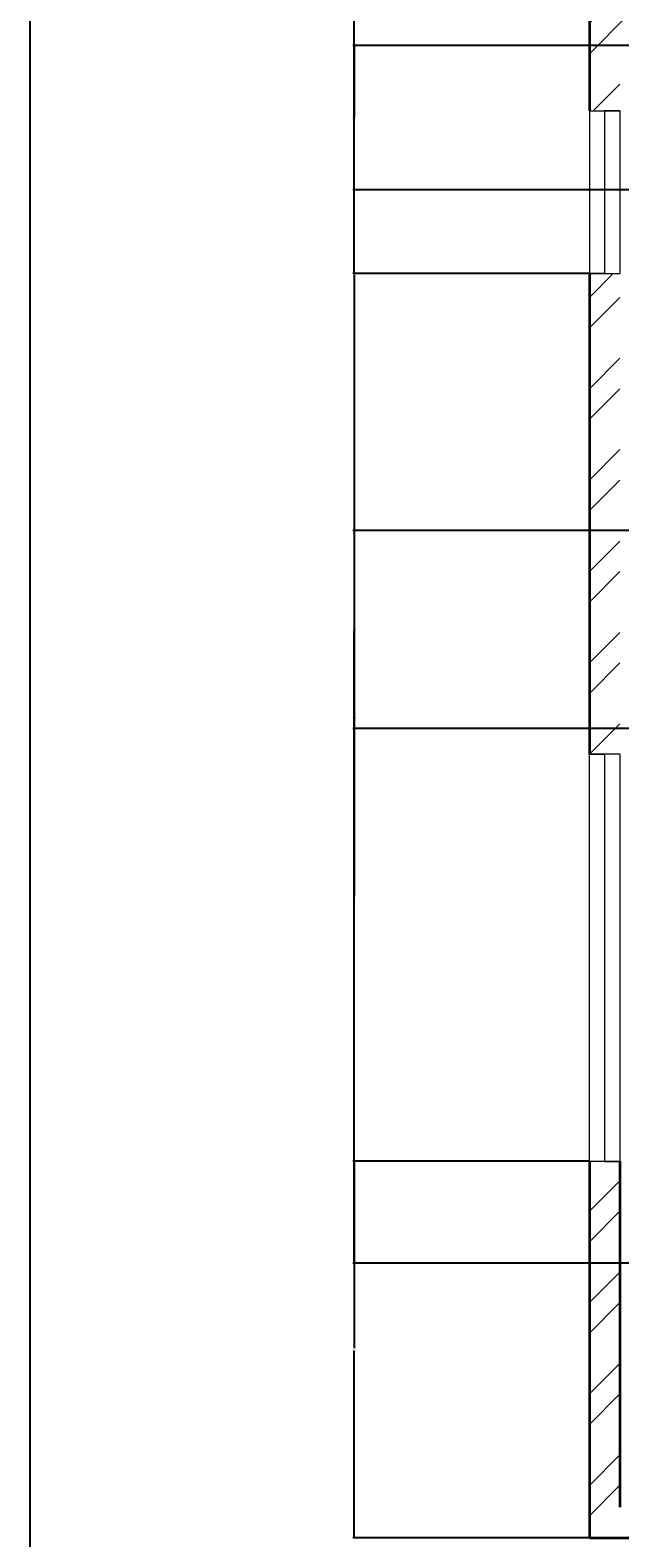
# Model space of a CAD drawing. Units: inches. Extents: x 1965 to 2673, y 1802 to 2669.
# Tile 2 of 16: x 1965 to 2052, y 1932 to 2154. Entities that reach past the tile are written whole.
import ezdxf

# ---------------------------------------------------------------- set-up
doc = ezdxf.new("R2010")
doc.units = ezdxf.units.IN
for name, color, linetype, lineweight in [('A-ANNO-DIMS', 2, 'Continuous', 18), ('A-ANNO-TTLB', 7, 'Continuous', 25), ('A-GLAZ', 181, 'Continuous', 18), ('A-WALL', 7, 'Continuous', 35), ('A-WALL-PATT', 252, 'Continuous', 13)]:
    doc.layers.add(name, color=color, linetype=linetype, lineweight=lineweight)
doc.styles.get("Standard").update_dxf_attribs({"font": 'arial.ttf'})
doc.dimstyles.get("Standard").update_dxf_attribs({"dimtxt": 0.18, "dimasz": 0.18, "dimexe": 0.18, "dimexo": 0.0625, "dimgap": 0.09, "dimtad": 0, "dimtih": 1, "dimtoh": 1, "dimdec": 4, "dimzin": 0, "dimdsep": 46, "dimtxsty": 'Standard', "dimcen": 0.09, "dimadec": 0, "dimazin": 0, "dimtfac": 1, "dimtdec": 4, "dimtofl": 0, "dimtmove": 0, "dimatfit": 3, "dimfxl": 1, "dimtolj": 1, "dimtzin": 0, "dimarcsym": 0})

# ---------------------------------------------------------------- blocks, each defined once
blk = doc.blocks.new('WIN-60IN')
for p, q in [((0, 4.5), (0, 0)), ((0, 4.5), (60, 4.5)), ((60, 2.25), (60, 4.5)), ((60, 4.5), (60, 0)), ((0, 0), (0, 2.25)), ((0, 2.25), (60, 2.25)), ((60, 0), (0, 0))]:
    blk.add_line(p, q)
blk = doc.blocks.new('WIN-24IN')
for p, q in [((0, 24), (4.5, 24)), ((0, 24), (0, 0)), ((4.5, 24), (2.25, 24)), ((2.25, 24), (2.25, 0)), ((4.5, 24), (4.5, 0)), ((2.25, 0), (0, 0)), ((0, 0), (4.5, 0))]:
    blk.add_line(p, q)
blk = doc.blocks.new('*D33')
at = {"layer": 'A-ANNO-DIMS', "color": 0, "lineweight": -2, "transparency": 16777216}
for p, q in [((2047.03, 1987.1), (2012.19, 1987.1)), ((2012.37, 1986.92), (2012.37, 1959.53)), ((2012.37, 1931.77), (2012.37, 1959.16)), ((2047.03, 1931.59), (2012.19, 1931.59))]:
    blk.add_line(p, q, dxfattribs=at)
at = {"layer": 'A-ANNO-DIMS', "color": 0, "transparency": 16777216}
for points in [[(2012.34, 1986.92), (2012.4, 1986.92), (2012.37, 1987.1)], [(2012.34, 1931.77), (2012.4, 1931.77), (2012.37, 1931.59)]]:
    blk.add_solid(points, dxfattribs=at)
at = {"layer": 'Defpoints', "color": 0, "transparency": 16777216}
for p in [(2012.37, 1987.1), (2047.09, 1987.1), (2047.09, 1931.59)]:
    blk.add_point(p, dxfattribs=at)
at = {"layer": 'A-ANNO-DIMS', "color": 0, "transparency": 16777216, "insert": (2012.37, 1959.34), "char_height": 0.18, "attachment_point": 5}
blk.add_mtext('\\A1;55.5', dxfattribs=at)
blk = doc.blocks.new('*D34')
at = {"layer": 'A-ANNO-DIMS', "color": 0, "lineweight": -2, "transparency": 16777216}
for p, q in [((2047.03, 2117.95), (2012.19, 2117.95)), ((2012.37, 2117.77), (2012.37, 2052.71)), ((2012.37, 1987.28), (2012.37, 2052.34)), ((2047.03, 1987.1), (2012.19, 1987.1))]:
    blk.add_line(p, q, dxfattribs=at)
at = {"layer": 'A-ANNO-DIMS', "color": 0, "transparency": 16777216}
for points in [[(2012.34, 2117.77), (2012.4, 2117.77), (2012.37, 2117.95)], [(2012.34, 1987.28), (2012.4, 1987.28), (2012.37, 1987.1)]]:
    blk.add_solid(points, dxfattribs=at)
at = {"layer": 'Defpoints', "color": 0, "transparency": 16777216}
for p in [(2012.37, 2117.95), (2047.09, 2117.95), (2047.09, 1987.1)]:
    blk.add_point(p, dxfattribs=at)
at = {"layer": 'A-ANNO-DIMS', "color": 0, "transparency": 16777216, "insert": (2012.37, 2052.52), "char_height": 0.18, "attachment_point": 5}
blk.add_mtext('\\A1;130.86', dxfattribs=at)
blk = doc.blocks.new('*D35')
at = {"layer": 'A-ANNO-DIMS', "color": 0, "lineweight": -2, "transparency": 16777216}
for p, q in [((2047.03, 2197.58), (2012.19, 2197.58)), ((2012.37, 2197.4), (2012.37, 2157.95)), ((2012.37, 2118.13), (2012.37, 2157.59)), ((2047.03, 2117.95), (2012.19, 2117.95))]:
    blk.add_line(p, q, dxfattribs=at)
at = {"layer": 'A-ANNO-DIMS', "color": 0, "transparency": 16777216}
for points in [[(2012.34, 2197.4), (2012.4, 2197.4), (2012.37, 2197.58)], [(2012.34, 2118.13), (2012.4, 2118.13), (2012.37, 2117.95)]]:
    blk.add_solid(points, dxfattribs=at)
at = {"layer": 'Defpoints', "color": 0, "transparency": 16777216}
for p in [(2012.37, 2197.58), (2047.09, 2197.58), (2047.09, 2117.95)]:
    blk.add_point(p, dxfattribs=at)
at = {"layer": 'A-ANNO-DIMS', "color": 0, "transparency": 16777216, "insert": (2012.37, 2157.77), "char_height": 0.18, "attachment_point": 5}
blk.add_mtext('\\A1;79.63', dxfattribs=at)
blk = doc.blocks.new('*D45')
at = {"layer": 'A-ANNO-DIMS', "color": 0, "lineweight": -2, "transparency": 16777216}
for p, q in [((2573.53, 2080.09), (2012.19, 2080.09)), ((2012.37, 2079.91), (2012.37, 2065.68)), ((2012.37, 2051.08), (2012.37, 2065.31)), ((2573.53, 2050.9), (2012.19, 2050.9))]:
    blk.add_line(p, q, dxfattribs=at)
at = {"layer": 'A-ANNO-DIMS', "color": 0, "transparency": 16777216}
for points in [[(2012.34, 2079.91), (2012.4, 2079.91), (2012.37, 2080.09)], [(2012.34, 2051.08), (2012.4, 2051.08), (2012.37, 2050.9)]]:
    blk.add_solid(points, dxfattribs=at)
at = {"layer": 'Defpoints', "color": 0, "transparency": 16777216}
for p in [(2012.37, 2080.09), (2573.59, 2080.09), (2573.59, 2050.9)]:
    blk.add_point(p, dxfattribs=at)
at = {"layer": 'A-ANNO-DIMS', "color": 0, "transparency": 16777216, "insert": (2012.37, 2065.49), "char_height": 0.18, "attachment_point": 5}
blk.add_mtext('\\A1;29.19', dxfattribs=at)
blk = doc.blocks.new('*D46')
at = {"layer": 'A-ANNO-DIMS', "color": 0, "lineweight": -2, "transparency": 16777216}
for p, q in [((2573.53, 2151.59), (2012.19, 2151.59)), ((2012.37, 2151.41), (2012.37, 2141.12)), ((2012.37, 2130.47), (2012.37, 2140.76)), ((2573.53, 2130.29), (2012.19, 2130.29))]:
    blk.add_line(p, q, dxfattribs=at)
at = {"layer": 'A-ANNO-DIMS', "color": 0, "transparency": 16777216}
for points in [[(2012.34, 2151.41), (2012.4, 2151.41), (2012.37, 2151.59)], [(2012.34, 2130.47), (2012.4, 2130.47), (2012.37, 2130.29)]]:
    blk.add_solid(points, dxfattribs=at)
at = {"layer": 'Defpoints', "color": 0, "transparency": 16777216}
for p in [(2012.37, 2151.59), (2573.59, 2151.59), (2573.59, 2130.29)]:
    blk.add_point(p, dxfattribs=at)
at = {"layer": 'A-ANNO-DIMS', "color": 0, "transparency": 16777216, "insert": (2012.37, 2140.94), "char_height": 0.18, "attachment_point": 5}
blk.add_mtext('\\A1;21.3', dxfattribs=at)
blk = doc.blocks.new('*D51')
at = {"layer": 'A-ANNO-DIMS', "color": 0, "lineweight": -2, "transparency": 16777216}
for p, q in [((2388.03, 2080.09), (2012.19, 2080.09)), ((2012.37, 2079.91), (2012.37, 2026.27)), ((2012.37, 1972.27), (2012.37, 2025.91)), ((2388.03, 1972.09), (2012.19, 1972.09))]:
    blk.add_line(p, q, dxfattribs=at)
at = {"layer": 'A-ANNO-DIMS', "color": 0, "transparency": 16777216}
for points in [[(2012.34, 2079.91), (2012.4, 2079.91), (2012.37, 2080.09)], [(2012.34, 1972.27), (2012.4, 1972.27), (2012.37, 1972.09)]]:
    blk.add_solid(points, dxfattribs=at)
at = {"layer": 'Defpoints', "color": 0, "transparency": 16777216}
for p in [(2012.37, 2080.09), (2388.09, 2080.09), (2388.09, 1972.09)]:
    blk.add_point(p, dxfattribs=at)
at = {"layer": 'A-ANNO-DIMS', "color": 0, "transparency": 16777216, "insert": (2012.37, 2026.09), "char_height": 0.18, "attachment_point": 5}
blk.add_mtext('\\A1;108', dxfattribs=at)

msp = doc.modelspace()

# ---------------------------------------------------------------- hatches: boundary and pattern name
at = {"layer": 'A-WALL-PATT'}
h = msp.add_hatch(dxfattribs=at)
h.set_pattern_fill('ANSI32', color=256)
h.paths.add_polyline_path([(2051.5927, 2561.0914), (2076.7559, 2561.0914), (2076.7559, 2563.3414), (2076.7559, 2565.5914), (2047.0927, 2565.5914), (2047.0927, 2518.3824), (2051.5927, 2518.3824)])
h.paths.add_polyline_path([(2051.5927, 2458.3824), (2049.3427, 2458.3824), (2047.0927, 2458.3824), (2047.0927, 2412.5914), (2248.0927, 2412.5914), (2248.0927, 2268.5914), (2252.5927, 2268.5914), (2252.5927, 2412.5914), (2252.5927, 2421.0404), (2250.3427, 2421.0404), (2248.0927, 2421.0404), (2248.0927, 2417.0914), (2051.5927, 2417.0914)])
h.paths.add_polyline_path([(2211.4933, 2268.5914), (2104.0927, 2268.5914), (2104.0927, 2272.4654), (2101.8427, 2272.4654), (2099.5927, 2272.4654), (2099.5927, 2268.5914), (2051.5927, 2268.5914), (2051.5927, 2264.0914), (2147.5927, 2264.0914), (2147.5927, 2259.8893), (2152.0927, 2259.8893), (2152.0927, 2264.0914), (2211.4933, 2264.0914), (2211.4933, 2266.3414)])
h.paths.add_polyline_path([(2104.0927, 2376.0914), (2099.5927, 2376.0914), (2047.0927, 2376.0914), (2047.0927, 2333.0682), (2051.5927, 2333.0682), (2051.5927, 2371.5914), (2099.5927, 2371.5914), (2099.5927, 2293.6123), (2104.0927, 2293.6123)], flags=17)
h.paths.add_polyline_path([(2051.5927, 2309.0682), (2047.0927, 2309.0682), (2047.0927, 2233.5821), (2051.5927, 2233.5821)])
h.paths.add_polyline_path([(2104.0927, 2412.5914), (2099.5927, 2412.5914), (2099.5927, 2376.0914), (2104.0927, 2376.0914)], flags=17)
h.paths.add_polyline_path([(2290.1254, 2268.5914), (2242.4924, 2268.5914), (2242.4924, 2264.0914), (2290.1254, 2264.0914), (2290.1254, 2266.3414)])
h.paths.add_polyline_path([(2284.653, 2264.0914), (2280.153, 2264.0914), (2280.153, 2161.6826), (2284.653, 2161.6826)])
h.paths.add_polyline_path([(2578.0927, 2329.4656), (2573.5927, 2329.4656), (2573.5927, 2268.5914), (2525.5927, 2268.5914), (2525.5927, 2271.9222), (2523.3427, 2271.9222), (2521.0927, 2271.9222), (2521.0927, 2268.5914), (2324.2835, 2268.5914), (2324.2835, 2264.0914), (2329.0927, 2264.0914), (2329.0927, 2259.4977), (2333.5927, 2259.4977), (2333.5927, 2264.0914), (2473.0927, 2264.0914), (2473.0927, 2259.9371), (2477.5927, 2259.9371), (2477.5927, 2264.0914), (2573.5927, 2264.0914), (2573.5927, 2235.5751), (2578.0927, 2235.5751)])
h.paths.add_polyline_path([(2377.0927, 2412.5914), (2578.0927, 2412.5914), (2578.0927, 2444.2286), (2575.8427, 2444.2286), (2573.5927, 2444.2286), (2573.5927, 2417.0914), (2429.5927, 2417.0914), (2377.0927, 2417.0914), (2377.0927, 2421.7443), (2372.5927, 2421.7443), (2372.5927, 2268.5914), (2377.0927, 2268.5914)])
h.paths.add_polyline_path([(2525.5927, 2371.5914), (2573.5927, 2371.5914), (2573.5927, 2353.4656), (2578.0927, 2353.4656), (2578.0927, 2376.0914), (2525.5927, 2376.0914), (2521.0927, 2376.0914), (2521.0927, 2290.6472), (2525.5927, 2290.6472)], flags=17)
h.paths.add_polyline_path([(2477.5927, 2236.4106), (2475.3427, 2236.4106), (2473.0927, 2236.4106), (2473.0927, 2084.5914), (2465.3309, 2084.5914), (2465.3309, 2080.0914), (2481.6764, 2080.0914), (2481.6764, 2082.3414), (2481.6764, 2084.5914), (2477.5927, 2084.5914), (2477.5927, 2151.5914), (2573.5927, 2151.5914), (2573.5927, 2130.2907), (2578.0927, 2130.2907), (2578.0927, 2199.5751), (2575.8427, 2199.5751), (2573.5927, 2199.5751), (2573.5927, 2156.0914), (2477.5927, 2156.0914)])
h.paths.add_polyline_path([(2573.5927, 2084.5914), (2505.5513, 2084.5914), (2505.5513, 2080.0914), (2573.5927, 2080.0914)], flags=17)
h.paths.add_polyline_path([(2578.0927, 2106.2907), (2575.8427, 2106.2907), (2573.5927, 2106.2907), (2573.5927, 2050.8986), (2578.0927, 2050.8986)])
h.paths.add_polyline_path([(2578.0927, 1990.8986), (2575.8427, 1990.8986), (2573.5927, 1990.8986), (2573.5927, 1936.0914), (2522.132, 1936.0914), (2522.132, 1931.5914), (2578.0927, 1931.5914)])
h.paths.add_polyline_path([(2462.132, 1936.0914), (2429.5927, 1936.0914), (2429.5927, 2080.0914), (2432.623, 2080.0914), (2432.623, 2082.3414), (2432.623, 2084.5914), (2429.5927, 2084.5914), (2429.5927, 2120.5914), (2333.5927, 2120.5914), (2333.5927, 2229.3125), (2331.3427, 2229.3125), (2329.0927, 2229.3125), (2329.0927, 2116.0914), (2425.0927, 2116.0914), (2425.0927, 1936.0914), (2346.4058, 1936.0914), (2346.4058, 1931.5914), (2462.132, 1931.5914), (2462.132, 1933.8414)])
h.paths.add_polyline_path([(2211.767, 1933.8414), (2211.767, 1936.0914), (2200.0927, 1936.0914), (2200.0927, 2080.0914), (2200.0927, 2116.0914), (2284.653, 2116.0914), (2284.653, 2130.591), (2282.403, 2130.591), (2280.153, 2130.591), (2280.153, 2120.5914), (2200.0927, 2120.5914), (2195.5927, 2120.5914), (2195.5927, 2080.0914), (2195.5927, 1936.0914), (2139.0533, 1936.0914), (2139.0533, 1931.5914), (2211.767, 1931.5914)])
h.paths.add_polyline_path([(2282.2502, 1933.8414), (2282.2502, 1936.0914), (2259.767, 1936.0914), (2259.767, 1931.5914), (2282.2502, 1931.5914)], flags=17)
h.paths.add_polyline_path([(2051.5927, 1987.096), (2049.3427, 1987.096), (2047.0927, 1987.096), (2047.0927, 1931.5914), (2079.0533, 1931.5914), (2079.0533, 1933.8414), (2079.0533, 1936.0914), (2051.5927, 1936.0914)])
h.paths.add_polyline_path([(2051.5927, 2197.5821), (2049.3427, 2197.5821), (2047.0927, 2197.5821), (2047.0927, 2141.952), (2051.5927, 2141.952), (2051.5927, 2151.5914), (2147.5927, 2151.5914), (2147.5927, 2084.5914), (2144.3652, 2084.5914), (2144.3652, 2080.0914), (2155.9662, 2080.0914), (2155.9662, 2082.3414), (2155.9662, 2084.5914), (2152.0927, 2084.5914), (2152.0927, 2239.4921), (2149.8427, 2239.4921), (2147.5927, 2239.4921), (2147.5927, 2156.0914), (2051.5927, 2156.0914)])
h.paths.add_polyline_path([(2051.5927, 2080.0914), (2123.8575, 2080.0914), (2123.8575, 2082.3414), (2123.8575, 2084.5914), (2051.5927, 2084.5914), (2051.5927, 2117.952), (2047.0927, 2117.952), (2047.0927, 2047.096), (2051.5927, 2047.096)])

# ---------------------------------------------------------------- linework, layer by layer
at = {"layer": 'A-ANNO-TTLB'}
msp.add_lwpolyline([(1964.5703, 2669.282), (2673.2605, 2669.282), (2673.2605, 1802.0221), (1964.5703, 1802.0221)], close=True, dxfattribs=at)
at = {"layer": 'A-WALL'}
for p, q in [((2047.0927, 2197.5821), (2047.0927, 2141.952)), ((2047.0927, 2117.952), (2047.0927, 2047.096)), ((2047.0927, 1987.096), (2047.0927, 1931.5914)), ((2051.5927, 1987.096), (2051.5927, 1936.0914)), ((2047.0927, 1931.5914), (2079.0533, 1931.5914))]:
    msp.add_line(p, q, dxfattribs=at)

# ---------------------------------------------------------------- block references
at = {"layer": 'A-GLAZ'}
msp.add_blockref('WIN-24IN', (2047.09, 2117.9563), dxfattribs=at)
at = {"layer": 'A-GLAZ', "rotation": 270}
msp.add_blockref('WIN-60IN', (2047.0913, 2047.0919), dxfattribs=at)

# ---------------------------------------------------------------- dimensions: what is measured, and where the dimension line sits
at = {"layer": 'A-ANNO-DIMS'}
for base, p1, p2, override, picture, middle in [((2012.3677, 2197.5821), (2047.0927, 2117.952), (2047.0927, 2197.5821), {"dimdec": 2, "dimlfac": 1, "dimrnd": 0, "dimzin": 0, "dimdsep": 46, "dimlunit": 2}, '*D35', (2012.3677, 2157.7671)), ((2012.3677, 2151.5914), (2573.5927, 2130.2907), (2573.5927, 2151.5914), {"dimdec": 1, "dimlfac": 1, "dimrnd": 0, "dimzin": 0, "dimdsep": 46, "dimlunit": 2}, '*D46', (2012.3677, 2140.941)), ((2012.3677, 2117.952), (2047.0927, 1987.096), (2047.0927, 2117.952), {"dimdec": 2, "dimlfac": 1, "dimrnd": 0, "dimzin": 0, "dimdsep": 46, "dimlunit": 2}, '*D34', (2012.3677, 2052.524)), ((2012.3677, 2080.0914), (2573.5927, 2050.8986), (2573.5927, 2080.0914), {"dimdec": 2, "dimlfac": 1, "dimrnd": 0, "dimzin": 0, "dimdsep": 46, "dimlunit": 2}, '*D45', (2012.3677, 2065.495)), ((2012.3677, 2080.0914), (2388.0925, 1972.0914), (2388.0925, 2080.0914), {"dimdec": 0, "dimlfac": 1, "dimrnd": 0, "dimzin": 0, "dimdsep": 46, "dimlunit": 2}, '*D51', (2012.3677, 2026.0914)), ((2012.3677, 1987.096), (2047.0927, 1931.5914), (2047.0927, 1987.096), {"dimdec": 1, "dimlfac": 1, "dimrnd": 0, "dimzin": 0, "dimdsep": 46, "dimlunit": 2}, '*D33', (2012.3677, 1959.3437))]:
    dim = msp.add_linear_dim(base=base, p1=p1, p2=p2, angle=90, dimstyle='Standard', override=override, dxfattribs=at)
    dim.commit()
    dim.dimension.update_dxf_attribs({"geometry": picture, "text_midpoint": middle})

doc.saveas('drawing.dxf')
